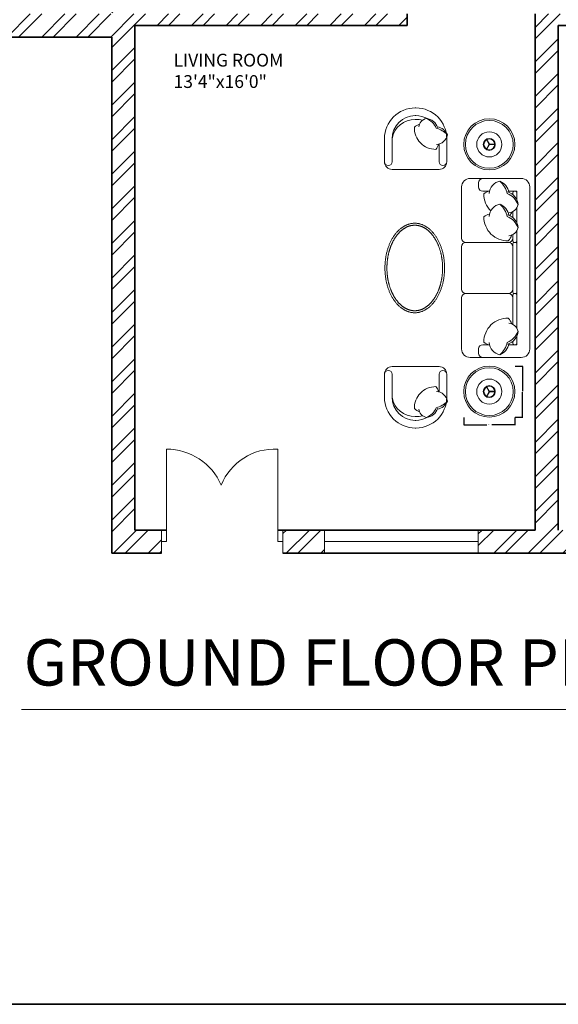
# Model space of a CAD drawing. Units: inches. Extents: x 1152 to 2588, y 1459 to 2618.
# Tile 2 of 17: x 1369 to 1579, y 1459 to 1843. Entities that reach past the tile are written whole.
import ezdxf

# ---------------------------------------------------------------- set-up
doc = ezdxf.new("R2010")
doc.units = ezdxf.units.IN
for name, color, linetype, lineweight in [('A-ANNO-DIMS', 2, 'Continuous', 18), ('A-ANNO-TEXT', 7, 'Continuous', 18), ('A-ANNO-TTLB', 7, 'Continuous', 35), ('A-AREA-IDEN', 7, 'Continuous', 18), ('A-DOOR', 4, 'Continuous', 18), ('A-FURN', 8, 'Continuous', 13), ('A-GLAZ', 4, 'Continuous', 18), ('A-WALL', 7, 'Continuous', 35), ('A-WALL-PATT', 8, 'Continuous', 13)]:
    doc.layers.add(name, color=color, linetype=linetype, lineweight=lineweight)
doc.styles.get("Standard").update_dxf_attribs({"font": 'arial.ttf'})
doc.dimstyles.get("Standard").update_dxf_attribs({"dimtxt": 0.18, "dimasz": 0.18, "dimexe": 0.18, "dimexo": 0.0625, "dimgap": 0.09, "dimtad": 0, "dimtih": 1, "dimtoh": 1, "dimdec": 4, "dimzin": 0, "dimdsep": 46, "dimtxsty": 'Standard', "dimcen": 0.09, "dimadec": 0, "dimazin": 0, "dimtfac": 1, "dimtdec": 4, "dimtofl": 0, "dimtmove": 0, "dimatfit": 3, "dimfxl": 1, "dimtolj": 1, "dimtzin": 0, "dimarcsym": 0})

# ---------------------------------------------------------------- blocks, each defined once
blk = doc.blocks.new('TABLE-ROUND-SIDE')
at = {"ltscale": 0.03}
for p, q in [((9.87, 9.91), (8.7, 11.94)), ((10.05, 10.01), (8.88, 12.04)), ((9.87, 10.01), (8.7, 7.99)), ((10.05, 9.91), (8.88, 7.88)), ((9.96, 10.07), (12.3, 10.07)), ((9.96, 9.86), (12.3, 9.86))]:
    blk.add_line(p, q, dxfattribs=at)
for radius in [9.96, 4.9, 2.34, 2.1]:
    blk.add_circle((9.96, 9.96), radius, dxfattribs=at)
blk.add_circle((9.96, 9.96), 9.3)
blk = doc.blocks.new('DOOR-DOUBLE-ENTRY')
for p, q in [((2, 4.5), (2, 40.5)), ((45.34, 4.5), (45.34, 40.5)), ((0, 9), (0, 0)), ((47.34, 9), (47.34, 0)), ((0, 0), (0, 4.5)), ((0, 4.5), (2, 4.5)), ((47.34, 4.5), (45.34, 4.5)), ((47.34, 0), (47.34, 4.5))]:
    blk.add_line(p, q)
for centre, radius, start, end in [((2, 17.3), 23.2, 23.3053, 90), ((44.08, 18.16), 22.37, 86.7789, 158.1829)]:
    blk.add_arc(centre, radius, start, end)
blk = doc.blocks.new('WIN-60-FRONT')
for p, q in [((0, 9), (0, 0)), ((60, 4.5), (60, 9)), ((60, 9), (60, 0)), ((0, 0), (0, 4.5)), ((0, 4.5), (48, 4.5)), ((48, 4.5), (60, 4.5))]:
    blk.add_line(p, q)
blk = doc.blocks.new('*D34')
at = {"layer": 'A-ANNO-DIMS', "color": 0, "lineweight": -2, "transparency": 16777216}
for p, q in [((1542.56, 1687.93), (1542.56, 1684.83)), ((1562.48, 1687.93), (1562.48, 1684.83)), ((1542.74, 1685.01), (1551.55, 1685.01)), ((1562.3, 1685.01), (1553.48, 1685.01))]:
    blk.add_line(p, q, dxfattribs=at)
at = {"layer": 'A-ANNO-DIMS', "color": 0, "transparency": 16777216}
for points in [[(1542.74, 1685.04), (1542.74, 1684.98), (1542.56, 1685.01)], [(1562.3, 1685.04), (1562.3, 1684.98), (1562.48, 1685.01)]]:
    blk.add_solid(points, dxfattribs=at)
at = {"layer": 'Defpoints', "color": 0, "transparency": 16777216}
for p in [(1542.56, 1688), (1562.48, 1688), (1562.48, 1685.01)]:
    blk.add_point(p, dxfattribs=at)
at = {"layer": 'A-ANNO-DIMS', "color": 0, "transparency": 16777216, "insert": (1552.52, 1685.01), "char_height": 0.18, "attachment_point": 5}
blk.add_mtext('\\A1;TABLE 20 TYP.', dxfattribs=at)
blk = doc.blocks.new('*D35')
at = {"layer": 'A-ANNO-DIMS', "color": 0, "lineweight": -2, "transparency": 16777216}
for p, q in [((1562.54, 1707.92), (1565.65, 1707.92)), ((1565.47, 1707.74), (1565.47, 1698.14)), ((1565.47, 1688.18), (1565.47, 1697.78)), ((1562.54, 1688), (1565.65, 1688))]:
    blk.add_line(p, q, dxfattribs=at)
at = {"layer": 'A-ANNO-DIMS', "color": 0, "transparency": 16777216}
for points in [[(1565.44, 1707.74), (1565.5, 1707.74), (1565.47, 1707.92)], [(1565.44, 1688.18), (1565.5, 1688.18), (1565.47, 1688)]]:
    blk.add_solid(points, dxfattribs=at)
at = {"layer": 'Defpoints', "color": 0, "transparency": 16777216}
for p in [(1562.48, 1707.92), (1565.47, 1707.92), (1562.48, 1688)]:
    blk.add_point(p, dxfattribs=at)
at = {"layer": 'A-ANNO-DIMS', "color": 0, "transparency": 16777216, "insert": (1565.47, 1697.96), "char_height": 0.18, "attachment_point": 5}
blk.add_mtext('\\A1;20 TYP.', dxfattribs=at)

msp = doc.modelspace()

# ---------------------------------------------------------------- hatches: boundary and pattern name
at = {"layer": 'A-WALL-PATT'}
h = msp.add_hatch(dxfattribs=at)
h.set_pattern_fill('ANSI32', color=256)
h.paths.add_polyline_path([(1408.9272, 2240.0458), (1276.4165, 2240.0458), (1276.4165, 2192.7491), (1285.4165, 2192.7491), (1285.4165, 2231.0458), (1369.4165, 2231.0458), (1369.4165, 2084.0458), (1526.9165, 2084.0458), (1526.9165, 2096.3728), (1524.6665, 2096.3728), (1522.4165, 2096.3728), (1522.4165, 2093.0458), (1378.4165, 2093.0458), (1378.4165, 2231.0458), (1408.9272, 2231.0458)])
h.paths.add_polyline_path([(1736.4165, 2240.0458), (1468.9272, 2240.0458), (1468.9272, 2231.0458), (1522.4165, 2231.0458), (1522.4165, 2127.3313), (1526.9165, 2127.3313), (1526.9165, 2231.0458), (1574.9165, 2231.0458), (1574.9165, 2188.0458), (1579.4165, 2188.0458), (1579.4165, 2231.0458), (1727.4165, 2231.0458), (1727.4165, 2183.9728), (1736.4165, 2183.9728)])
h.paths.add_polyline_path([(1285.4165, 2156.7491), (1276.4165, 2156.7491), (1276.4165, 2084.0458), (1285.4165, 2084.0458)], flags=17)
h.paths.add_polyline_path([(1285.4165, 2043.5458), (1445.4165, 2043.5458), (1445.4165, 1943.6503), (1454.4165, 1943.6503), (1454.4165, 2048.0458), (1276.4165, 2048.0458), (1276.4165, 2019.2077), (1280.9165, 2019.2077), (1285.4165, 2019.2077)])
h.paths.add_polyline_path([(1285.4165, 1959.2077), (1276.4165, 1959.2077), (1276.4165, 1891.1319), (1280.9165, 1891.1319), (1285.4165, 1891.1319), (1285.4165, 1901.0458), (1376.8505, 1901.0458), (1376.8505, 1903.2958), (1376.8505, 1905.5458), (1285.4165, 1905.5458)])
h.paths.add_polyline_path([(1518.4165, 1905.5458), (1399.2832, 1905.5458), (1399.2832, 1903.2958), (1399.2832, 1901.0458), (1405.4165, 1901.0458), (1405.4165, 1884.8579), (1409.9165, 1884.8579), (1409.9165, 1901.0458), (1513.9165, 1901.0458), (1513.9165, 1869.1706), (1518.4165, 1869.1706)])
h.paths.add_polyline_path([(1520.5229, 1845.0458), (1518.4165, 1845.0458), (1518.4165, 1849.2927), (1516.1665, 1849.2927), (1513.9165, 1849.2927), (1513.9165, 1845.0458), (1409.9165, 1845.0458), (1409.9165, 1860.8579), (1405.4165, 1860.8579), (1405.4165, 1845.0458), (1285.4165, 1845.0458), (1285.4165, 1867.1319), (1276.4165, 1867.1319), (1276.4165, 1635.0458), (1285.4165, 1635.0458), (1285.4165, 1836.0458), (1405.4165, 1836.0458), (1405.4165, 1635.0458), (1414.4165, 1635.0458), (1424.7277, 1635.0458), (1424.7277, 1639.5458), (1424.7277, 1644.0458), (1414.4165, 1644.0458), (1414.4165, 1836.0458), (1414.4165, 1840.5831), (1520.5229, 1840.5831)])
h.paths.add_polyline_path([(1579.4165, 1840.5458), (1583.4035, 1840.5458), (1583.4035, 1845.0458), (1579.4165, 1845.0458), (1570.4165, 1845.0458), (1570.4165, 1840.5831), (1570.4165, 1644.0458), (1548.2359, 1644.0458), (1548.2359, 1635.0458), (1611.2801, 1635.0458), (1611.2801, 1639.5458), (1611.2801, 1644.0458), (1579.4165, 1644.0458)])
h.paths.add_polyline_path([(1488.2359, 1644.0458), (1472.0663, 1644.0458), (1472.0663, 1635.0458), (1488.2359, 1635.0458), (1488.2359, 1639.5458)], flags=17)
h.paths.add_polyline_path([(1736.4165, 1701.1863), (1727.4165, 1701.1863), (1727.4165, 1644.0458), (1671.2801, 1644.0458), (1671.2801, 1635.0458), (1736.4165, 1635.0458)])
h.paths.add_polyline_path([(1736.4165, 2147.9728), (1727.4165, 2147.9728), (1727.4165, 2093.0458), (1579.4165, 2093.0458), (1574.9165, 2093.0458), (1574.9165, 1971.6501), (1579.4165, 1971.6501), (1579.4165, 2084.0458), (1727.4165, 2084.0458), (1727.4165, 2054.3847), (1736.4165, 2054.3847)])
h.paths.add_polyline_path([(1736.4165, 1994.3847), (1727.4165, 1994.3847), (1727.4165, 1911.3562), (1736.4165, 1911.3562)])
h.paths.add_polyline_path([(1736.4165, 1875.3562), (1727.4165, 1875.3562), (1727.4165, 1845.0458), (1617.1767, 1845.0458), (1617.1767, 1842.7958), (1617.1767, 1840.5458), (1618.9165, 1840.5458), (1618.9165, 1788.5458), (1618.9165, 1784.0458), (1627.8699, 1784.0458), (1627.8699, 1788.5458), (1623.4165, 1788.5458), (1623.4165, 1840.5458), (1727.4165, 1840.5458), (1727.4165, 1828.7619), (1736.4165, 1828.7619)])
h.paths.add_polyline_path([(1727.4165, 1938.0458), (1579.4165, 1938.0458), (1579.4165, 1942.7722), (1574.9165, 1942.7722), (1574.9165, 1929.0458), (1727.4165, 1929.0458)])

# ---------------------------------------------------------------- linework, layer by layer
at = {"layer": 'A-ANNO-TEXT'}
msp.add_line((1370.1295, 1574.1335), (1649.1589, 1574.1335), dxfattribs=at)
at = {"layer": 'A-ANNO-TTLB'}
msp.add_lwpolyline([(1152.3215, 2617.6685), (2587.6987, 2617.6685), (2587.6987, 1459.3148), (1152.3215, 1459.3148)], close=True, dxfattribs=at)
at = {"layer": 'A-FURN', "ltscale": 0.03}
for points in [[(1523.795, 1784.4921), (1514.6636, 1784.4921, -0.41421356), (1511.6697, 1787.486), (1511.6697, 1796.4677, -0.41421356), (1523.6453, 1808.4434), (1523.795, 1808.4434), (1523.9447, 1808.4434, -0.41421356), (1535.9204, 1796.4677), (1535.9204, 1787.486, -0.41421356), (1532.9265, 1784.4921), (1523.795, 1784.4921)], [(1523.795, 1707.7174), (1514.6636, 1707.7174, 0.41421356), (1511.6697, 1704.7235), (1511.6697, 1695.7417, 0.41421356), (1523.6453, 1683.7661), (1523.795, 1683.7661), (1523.9447, 1683.7661, 0.41421356), (1535.9204, 1695.7417), (1535.9204, 1704.7235, 0.41421356), (1532.9265, 1707.7174), (1523.795, 1707.7174)]]:
    msp.add_lwpolyline(points, format="xyb", dxfattribs=at)
at = {"layer": 'A-FURN'}
for points in [[(1514.6636, 1796.4677, -0.41421356), (1523.6453, 1805.4495), (1523.795, 1805.4495)], [(1514.6636, 1796.4677, -0.37271891), (1523.6453, 1803.9525), (1523.795, 1803.9525)], [(1528.4031, 1804.2648, 0.13059149), (1523.9447, 1805.4495), (1523.795, 1805.4495)], [(1526.4969, 1803.63, 0.07238424), (1523.9447, 1803.9525), (1523.795, 1803.9525)], [(1532.3945, 1800.7566, 0.30666349), (1527.9296, 1804.3248, 0.30632997), (1525.0128, 1801.0661, -0.87284716)], [(1536.1652, 1797.9789, 0.14772988), (1531.7901, 1800.5515, 0.21334276), (1527.9296, 1804.3248, 0.17866181)], [(1532.6303, 1794.2969, -0.16554063), (1531.7043, 1792.319, -0.42598917), (1523.2971, 1800.8945, -0.12152332), (1525.2928, 1802.0765, 7.11546429)], [(1531.8758, 1794.2056, 0.35677236), (1536.1652, 1797.9789, 0.24954205), (1532.2786, 1801.0883, -9.61688035)], [(1514.6636, 1796.4679), (1514.6636, 1787.486, -0.41421356), (1513.1666, 1785.989), (1513.1666, 1785.989, -0.41421356), (1511.6697, 1787.486)], [(1532.9265, 1794.3689), (1532.9265, 1787.486, 0.41421356), (1534.4234, 1785.989), (1534.4234, 1785.989, 0.41421356), (1535.9204, 1787.486)], [(1552.5995, 1775.9894), (1550.0272, 1775.9894, -0.41421356), (1548.3669, 1777.6497), (1548.3669, 1779.31, -0.41421356), (1550.0272, 1780.9702)], [(1552.499, 1775.1563, -0.35677236), (1556.6839, 1779.9136, -0.24954205), (1560.1326, 1775.603, 9.61688035)], [(1556.6839, 1779.9136, -0.14772988), (1559.5372, 1775.0611, -0.21334276), (1563.7221, 1770.7795, -0.17866181)], [(1552.6003, 1775.9931, 0.16554063), (1550.4066, 1774.966, 0.20023115), (1553.0783, 1768.3753, 0.12152332)], [(1559.7646, 1775.7315, -0.30666349), (1563.7221, 1770.7795, -0.30632997), (1560.1079, 1767.5445, 0.87284716)], [(1563.3092, 1772.4967), (1563.3092, 1775.9894), (1560.0464, 1775.9894, -0.41421356)], [(1561.649, 1774.7225), (1561.649, 1775.3253, -0.41421356), (1562.3131, 1775.9894), (1562.6451, 1775.9894, -0.41421356), (1563.3092, 1775.3253)], [(1563.3092, 1775.3253), (1563.3092, 1772.4967, -0.41421356)], [(1552.499, 1766.2125, -0.35677236), (1556.6839, 1770.9698, -0.24954205), (1560.1326, 1766.6592, 9.61688035)], [(1556.6839, 1770.9698, -0.14772988), (1559.5372, 1766.1173, -0.21334276), (1563.7221, 1761.8358, -0.17866181)], [(1561.649, 1765.7787), (1561.649, 1768.0629, -0.41421356)], [(1563.3092, 1769.7346), (1563.3092, 1763.5529, -0.41421356)], [(1552.6003, 1767.0493, 0.16554063), (1550.4066, 1766.0222, 0.42598917), (1559.9177, 1756.6978, 0.12152332), (1561.2286, 1758.9113, -7.11546429)], [(1559.7646, 1766.7877, -0.30666349), (1563.7221, 1761.8358, -0.30632997), (1560.1079, 1758.6008, 0.87284716)], [(1560.5795, 1766.4631, 0.07186538), (1561.2286, 1767.855, -7.11546429)], [(1563.3092, 1760.7909), (1563.3092, 1756.7304, -0.41421356), (1562.6451, 1756.0663), (1562.3131, 1756.0663, -0.41421356), (1561.649, 1756.7304), (1561.649, 1759.1191, -0.41421356)], [(1561.649, 1757.7266, -0.41421356), (1559.9887, 1756.0663), (1543.3861, 1756.0663, -0.41421356)], [(1561.649, 1754.406, 0.41421356), (1559.9887, 1756.0663)], [(1561.649, 1737.8034, -0.41421356), (1559.9887, 1736.1432)], [(1561.649, 1734.4829, 0.41421356), (1559.9887, 1736.1432), (1543.3861, 1736.1432, 0.41421356)], [(1563.3092, 1722.4748), (1563.3092, 1735.4791, 0.41421356), (1562.6451, 1736.1432), (1562.3131, 1736.1432, 0.41421356), (1561.649, 1735.4791), (1561.649, 1724.1466, 0.41421356)], [(1552.6003, 1716.2164, -0.16554063), (1550.4066, 1717.2435, -0.42598917), (1559.9177, 1726.5679, -0.12152332), (1561.2286, 1724.3544, 7.11546429)], [(1559.7646, 1716.478, 0.30666349), (1563.7221, 1721.43, 0.30632997), (1560.1079, 1724.6649, -0.87284716)], [(1556.6839, 1712.2959, 0.14772988), (1559.5372, 1717.1484, 0.21334276), (1563.7221, 1721.43, 0.17866181)], [(1563.3092, 1716.8841), (1563.3092, 1719.7128, 0.41421356)], [(1550.0272, 1711.2392, -0.41421356), (1548.3669, 1712.8995), (1548.3669, 1714.5598, -0.41421356), (1550.0272, 1716.22), (1552.5995, 1716.22)], [(1552.499, 1717.0532, 0.35677236), (1556.6839, 1712.2959, 0.24954205), (1560.1326, 1716.6065, -9.61688035)], [(1561.649, 1717.487), (1561.649, 1716.8841, 0.41421356), (1562.3131, 1716.22), (1562.6451, 1716.22, 0.41421356), (1563.3092, 1716.8841)], [(1514.6636, 1695.7416), (1514.6636, 1704.7235, 0.41421356), (1513.1666, 1706.2204), (1513.1666, 1706.2204, 0.41421356), (1511.6697, 1704.7235)], [(1532.9265, 1697.8406), (1532.9265, 1704.7235, -0.41421356), (1534.4234, 1706.2204), (1534.4234, 1706.2204, -0.41421356), (1535.9204, 1704.7235)], [(1532.6303, 1697.9126, 0.16554063), (1531.7043, 1699.8905, 0.42598917), (1523.2971, 1691.3149, 0.12152332), (1525.2928, 1690.1329, -7.11546429)], [(1514.6636, 1695.7417, 0.37271891), (1523.6453, 1688.257), (1523.795, 1688.257)], [(1514.6636, 1695.7417, 0.41421356), (1523.6453, 1686.76), (1523.795, 1686.76)], [(1531.8758, 1698.0039, -0.35677236), (1536.1652, 1694.2306, -0.24954205), (1532.2786, 1691.1211, 9.61688035)], [(1532.3945, 1691.4529, -0.30666349), (1527.9296, 1687.8847, -0.30632997), (1525.0128, 1691.1434, 0.87284716)], [(1536.1652, 1694.2306, -0.14772988), (1531.7901, 1691.6579, -0.21334276), (1527.9296, 1687.8847, -0.17866181)], [(1526.4969, 1688.5795, -0.07238424), (1523.9447, 1688.257), (1523.795, 1688.257)], [(1528.4031, 1687.9446, -0.13059149), (1523.9447, 1686.76), (1523.795, 1686.76)]]:
    msp.add_lwpolyline(points, format="xyb", dxfattribs=at)
at = {"layer": 'A-FURN', "ltscale": 0.03}
msp.add_lwpolyline([(1545.0464, 1711.2392, -0.41421356), (1541.7258, 1714.5598), (1541.7258, 1734.4829, -0.41421356), (1543.3861, 1736.1432, -0.41421356), (1541.7258, 1737.8034), (1541.7258, 1754.406, -0.41421356), (1543.3861, 1756.0663, -0.41421356), (1541.7258, 1757.7266), (1541.7258, 1777.6497, -0.41421356), (1545.0464, 1780.9702), (1564.9695, 1780.9702, -0.41421356), (1568.29, 1777.6497), (1568.29, 1714.5598, -0.41421356), (1564.9695, 1711.2392)], format="xyb", close=True, dxfattribs=at)
at = {"layer": 'A-FURN'}
for points in [[(1563.3092, 1763.5529), (1563.3092, 1769.7346)], [(1563.3092, 1722.4748), (1563.3092, 1760.7909)], [(1560.0464, 1716.22), (1563.3092, 1716.22), (1563.3092, 1719.7128)]]:
    msp.add_lwpolyline(points, dxfattribs=at)
msp.add_lwpolyline([(1563.3092, 1755.4022), (1563.3092, 1736.8073, -0.41421356), (1562.6451, 1736.1432), (1562.3131, 1736.1432, -0.41421356), (1561.649, 1736.8073), (1561.649, 1755.4022, -0.41421356), (1562.3131, 1756.0663), (1562.6451, 1756.0663, -0.41421356)], format="xyb", close=True, dxfattribs=at)
at = {"layer": 'A-FURN', "ltscale": 0.03}
msp.add_polyline3d([(1523.463, 1728.672, 0), (1523.6829, 1728.6751, 0), (1523.9028, 1728.6845, 0), (1524.1225, 1728.7001, 0), (1524.3419, 1728.7219, 0), (1524.5611, 1728.75, 0), (1524.7798, 1728.7843, 0), (1524.9981, 1728.8247, 0), (1525.2158, 1728.8714, 0), (1525.4329, 1728.9243, 0), (1525.6493, 1728.9833, 0), (1525.8649, 1729.0484, 0), (1526.0797, 1729.1196, 0), (1526.2935, 1729.1969, 0), (1526.5063, 1729.2803, 0), (1526.718, 1729.3697, 0), (1526.9286, 1729.4651, 0), (1527.1379, 1729.5665, 0), (1527.3459, 1729.6737, 0), (1527.5525, 1729.7869, 0), (1527.7576, 1729.9059, 0), (1527.9612, 1730.0307, 0), (1528.1632, 1730.1613, 0), (1528.3635, 1730.2976, 0), (1528.562, 1730.4395, 0), (1528.7588, 1730.5871, 0), (1528.9536, 1730.7402, 0), (1529.1464, 1730.8988, 0), (1529.3373, 1731.0628, 0), (1529.526, 1731.2323, 0), (1529.7125, 1731.407, 0), (1529.8968, 1731.5871, 0), (1530.0788, 1731.7723, 0), (1530.2585, 1731.9627, 0), (1530.4357, 1732.1581, 0), (1530.6104, 1732.3585, 0), (1530.7825, 1732.5639, 0), (1530.952, 1732.7741, 0), (1531.1189, 1732.989, 0), (1531.283, 1733.2087, 0), (1531.4443, 1733.433, 0), (1531.6027, 1733.6618, 0), (1531.7582, 1733.8951, 0), (1531.9108, 1734.1328, 0), (1532.0603, 1734.3747, 0), (1532.2068, 1734.6209, 0), (1532.3501, 1734.8711, 0), (1532.4902, 1735.1254, 0), (1532.6271, 1735.3836, 0), (1532.7607, 1735.6457, 0), (1532.891, 1735.9115, 0), (1533.0179, 1736.1809, 0), (1533.1414, 1736.4539, 0), (1533.2614, 1736.7304, 0), (1533.378, 1737.0102, 0), (1533.4909, 1737.2933, 0), (1533.6003, 1737.5795, 0), (1533.706, 1737.8688, 0), (1533.8081, 1738.1611, 0), (1533.9065, 1738.4561, 0), (1534.0011, 1738.754, 0), (1534.0919, 1739.0544, 0), (1534.179, 1739.3574, 0), (1534.2622, 1739.6628, 0), (1534.3415, 1739.9705, 0), (1534.417, 1740.2804, 0), (1534.4885, 1740.5924, 0), (1534.5561, 1740.9063, 0), (1534.6197, 1741.2222, 0), (1534.6793, 1741.5397, 0), (1534.7348, 1741.8589, 0), (1534.7864, 1742.1797, 0), (1534.8339, 1742.5018, 0), (1534.8773, 1742.8252, 0), (1534.9166, 1743.1498, 0), (1534.9519, 1743.4755, 0), (1534.983, 1743.8021, 0), (1535.01, 1744.1295, 0), (1535.0328, 1744.4576, 0), (1535.0515, 1744.7863, 0), (1535.0661, 1745.1155, 0), (1535.0765, 1745.4451, 0), (1535.0827, 1745.7748, 0), (1535.0848, 1746.1047, 0), (1535.0827, 1746.4346, 0), (1535.0765, 1746.7644, 0), (1535.0661, 1747.094, 0), (1535.0515, 1747.4232, 0), (1535.0328, 1747.7519, 0), (1535.01, 1748.08, 0), (1534.983, 1748.4074, 0), (1534.9519, 1748.734, 0), (1534.9166, 1749.0597, 0), (1534.8773, 1749.3843, 0), (1534.8339, 1749.7077, 0), (1534.7864, 1750.0298, 0), (1534.7348, 1750.3505, 0), (1534.6793, 1750.6698, 0), (1534.6197, 1750.9873, 0), (1534.5561, 1751.3031, 0), (1534.4885, 1751.6171, 0), (1534.417, 1751.9291, 0), (1534.3415, 1752.239, 0), (1534.2622, 1752.5467, 0), (1534.179, 1752.8521, 0), (1534.0919, 1753.1551, 0), (1534.0011, 1753.4555, 0), (1533.9065, 1753.7533, 0), (1533.8081, 1754.0484, 0), (1533.706, 1754.3407, 0), (1533.6003, 1754.6299, 0), (1533.4909, 1754.9162, 0), (1533.378, 1755.1993, 0), (1533.2614, 1755.4791, 0), (1533.1414, 1755.7555, 0), (1533.0179, 1756.0285, 0), (1532.891, 1756.298, 0), (1532.7607, 1756.5638, 0), (1532.6271, 1756.8258, 0), (1532.4902, 1757.0841, 0), (1532.3501, 1757.3383, 0), (1532.2068, 1757.5886, 0), (1532.0603, 1757.8348, 0), (1531.9108, 1758.0767, 0), (1531.7582, 1758.3144, 0), (1531.6027, 1758.5476, 0), (1531.4443, 1758.7765, 0), (1531.283, 1759.0008, 0), (1531.1189, 1759.2204, 0), (1530.952, 1759.4354, 0), (1530.7825, 1759.6456, 0), (1530.6104, 1759.8509, 0), (1530.4357, 1760.0514, 0), (1530.2585, 1760.2468, 0), (1530.0788, 1760.4372, 0), (1529.8968, 1760.6224, 0), (1529.7125, 1760.8024, 0), (1529.526, 1760.9772, 0), (1529.3373, 1761.1466, 0), (1529.1464, 1761.3107, 0), (1528.9536, 1761.4693, 0), (1528.7588, 1761.6224, 0), (1528.562, 1761.77, 0), (1528.3635, 1761.9119, 0), (1528.1632, 1762.0482, 0), (1527.9612, 1762.1787, 0), (1527.7576, 1762.3036, 0), (1527.5525, 1762.4226, 0), (1527.3459, 1762.5357, 0), (1527.1379, 1762.643, 0), (1526.9286, 1762.7444, 0), (1526.718, 1762.8398, 0), (1526.5063, 1762.9292, 0), (1526.2935, 1763.0125, 0), (1526.0797, 1763.0899, 0), (1525.8649, 1763.1611, 0), (1525.6493, 1763.2262, 0), (1525.4329, 1763.2852, 0), (1525.2158, 1763.3381, 0), (1524.9981, 1763.3847, 0), (1524.7798, 1763.4252, 0), (1524.5611, 1763.4595, 0), (1524.3419, 1763.4876, 0), (1524.1225, 1763.5094, 0), (1523.9028, 1763.525, 0), (1523.6829, 1763.5344, 0), (1523.463, 1763.5375, 0), (1523.243, 1763.5344, 0), (1523.0232, 1763.525, 0), (1522.8035, 1763.5094, 0), (1522.584, 1763.4876, 0), (1522.3649, 1763.4595, 0), (1522.1461, 1763.4252, 0), (1521.9279, 1763.3847, 0), (1521.7101, 1763.3381, 0), (1521.493, 1763.2852, 0), (1521.2766, 1763.2262, 0), (1521.061, 1763.1611, 0), (1520.8463, 1763.0899, 0), (1520.6324, 1763.0125, 0), (1520.4196, 1762.9292, 0), (1520.2079, 1762.8398, 0), (1519.9974, 1762.7444, 0), (1519.7881, 1762.643, 0), (1519.5801, 1762.5357, 0), (1519.3735, 1762.4226, 0), (1519.1683, 1762.3036, 0), (1518.9647, 1762.1787, 0), (1518.7628, 1762.0482, 0), (1518.5625, 1761.9119, 0), (1518.3639, 1761.77, 0), (1518.1672, 1761.6224, 0), (1517.9724, 1761.4693, 0), (1517.7795, 1761.3107, 0), (1517.5887, 1761.1466, 0), (1517.4, 1760.9772, 0), (1517.2134, 1760.8024, 0), (1517.0291, 1760.6224, 0), (1516.8471, 1760.4372, 0), (1516.6675, 1760.2468, 0), (1516.4903, 1760.0514, 0), (1516.3156, 1759.8509, 0), (1516.1434, 1759.6456, 0), (1515.9739, 1759.4354, 0), (1515.8071, 1759.2204, 0), (1515.643, 1759.0008, 0), (1515.4817, 1758.7765, 0), (1515.3232, 1758.5476, 0), (1515.1677, 1758.3144, 0), (1515.0152, 1758.0767, 0), (1514.8656, 1757.8348, 0), (1514.7192, 1757.5886, 0), (1514.5759, 1757.3383, 0), (1514.4357, 1757.0841, 0), (1514.2988, 1756.8258, 0), (1514.1652, 1756.5638, 0), (1514.0349, 1756.298, 0), (1513.908, 1756.0285, 0), (1513.7845, 1755.7555, 0), (1513.6645, 1755.4791, 0), (1513.548, 1755.1993, 0), (1513.435, 1754.9162, 0), (1513.3257, 1754.6299, 0), (1513.2199, 1754.3407, 0), (1513.1179, 1754.0484, 0), (1513.0195, 1753.7533, 0), (1512.9249, 1753.4555, 0), (1512.834, 1753.1551, 0), (1512.747, 1752.8521, 0), (1512.6638, 1752.5467, 0), (1512.5844, 1752.239, 0), (1512.509, 1751.9291, 0), (1512.4375, 1751.6171, 0), (1512.3699, 1751.3031, 0), (1512.3063, 1750.9873, 0), (1512.2467, 1750.6698, 0), (1512.1911, 1750.3505, 0), (1512.1396, 1750.0298, 0), (1512.0921, 1749.7077, 0), (1512.0487, 1749.3843, 0), (1512.0093, 1749.0597, 0), (1511.9741, 1748.734, 0), (1511.943, 1748.4074, 0), (1511.916, 1748.08, 0), (1511.8931, 1747.7519, 0), (1511.8744, 1747.4232, 0), (1511.8599, 1747.094, 0), (1511.8495, 1746.7644, 0), (1511.8432, 1746.4346, 0), (1511.8411, 1746.1047, 0), (1511.8432, 1745.7748, 0), (1511.8495, 1745.4451, 0), (1511.8599, 1745.1155, 0), (1511.8744, 1744.7863, 0), (1511.8931, 1744.4576, 0), (1511.916, 1744.1295, 0), (1511.943, 1743.8021, 0), (1511.9741, 1743.4755, 0), (1512.0093, 1743.1498, 0), (1512.0487, 1742.8252, 0), (1512.0921, 1742.5018, 0), (1512.1396, 1742.1797, 0), (1512.1911, 1741.8589, 0), (1512.2467, 1741.5397, 0), (1512.3063, 1741.2222, 0), (1512.3699, 1740.9063, 0), (1512.4375, 1740.5924, 0), (1512.509, 1740.2804, 0), (1512.5844, 1739.9705, 0), (1512.6638, 1739.6628, 0), (1512.747, 1739.3574, 0), (1512.834, 1739.0544, 0), (1512.9249, 1738.754, 0), (1513.0195, 1738.4561, 0), (1513.1179, 1738.1611, 0), (1513.2199, 1737.8688, 0), (1513.3257, 1737.5795, 0), (1513.435, 1737.2933, 0), (1513.548, 1737.0102, 0), (1513.6645, 1736.7304, 0), (1513.7845, 1736.4539, 0), (1513.908, 1736.1809, 0), (1514.0349, 1735.9115, 0), (1514.1652, 1735.6457, 0), (1514.2988, 1735.3836, 0), (1514.4357, 1735.1254, 0), (1514.5759, 1734.8711, 0), (1514.7192, 1734.6209, 0), (1514.8656, 1734.3747, 0), (1515.0152, 1734.1328, 0), (1515.1677, 1733.8951, 0), (1515.3232, 1733.6618, 0), (1515.4817, 1733.433, 0), (1515.643, 1733.2087, 0), (1515.8071, 1732.989, 0), (1515.9739, 1732.7741, 0), (1516.1434, 1732.5639, 0), (1516.3156, 1732.3585, 0), (1516.4903, 1732.1581, 0), (1516.6675, 1731.9627, 0), (1516.8471, 1731.7723, 0), (1517.0291, 1731.5871, 0), (1517.2134, 1731.407, 0), (1517.4, 1731.2323, 0), (1517.5887, 1731.0628, 0), (1517.7795, 1730.8988, 0), (1517.9724, 1730.7402, 0), (1518.1672, 1730.5871, 0), (1518.3639, 1730.4395, 0), (1518.5625, 1730.2976, 0), (1518.7628, 1730.1613, 0), (1518.9647, 1730.0307, 0), (1519.1683, 1729.9059, 0), (1519.3735, 1729.7869, 0), (1519.5801, 1729.6737, 0), (1519.7881, 1729.5665, 0), (1519.9974, 1729.4651, 0), (1520.2079, 1729.3697, 0), (1520.4196, 1729.2803, 0), (1520.6324, 1729.1969, 0), (1520.8463, 1729.1196, 0), (1521.061, 1729.0484, 0), (1521.2766, 1728.9833, 0), (1521.493, 1728.9243, 0), (1521.7101, 1728.8714, 0), (1521.9279, 1728.8247, 0), (1522.1461, 1728.7843, 0), (1522.3649, 1728.75, 0), (1522.584, 1728.7219, 0), (1522.8035, 1728.7001, 0), (1523.0232, 1728.6845, 0), (1523.243, 1728.6751, 0), (1523.463, 1728.672, 0)], dxfattribs=at)
at = {"layer": 'A-FURN'}
msp.add_polyline3d([(1523.463, 1729.4468, 0), (1523.5818, 1729.4478, 0), (1523.7012, 1729.4509, 0), (1523.8212, 1729.456, 0), (1523.9416, 1729.4632, 0), (1524.0626, 1729.4726, 0), (1524.184, 1729.4841, 0), (1524.3059, 1729.4978, 0), (1524.4283, 1729.5138, 0), (1524.551, 1729.5319, 0), (1524.6742, 1729.5523, 0), (1524.7978, 1729.575, 0), (1524.9218, 1729.6001, 0), (1525.0462, 1729.6274, 0), (1525.1709, 1729.6572, 0), (1525.2959, 1729.6893, 0), (1525.4212, 1729.7239, 0), (1525.5469, 1729.7609, 0), (1525.6728, 1729.8004, 0), (1525.799, 1729.8424, 0), (1525.9254, 1729.8869, 0), (1526.0521, 1729.934, 0), (1526.179, 1729.9837, 0), (1526.306, 1730.036, 0), (1526.4331, 1730.091, 0), (1526.5604, 1730.1486, 0), (1526.6876, 1730.2089, 0), (1526.8149, 1730.2717, 0), (1526.9421, 1730.3373, 0), (1527.0693, 1730.4055, 0), (1527.1964, 1730.4763, 0), (1527.3233, 1730.5498, 0), (1527.45, 1730.626, 0), (1527.5765, 1730.7048, 0), (1527.7028, 1730.7863, 0), (1527.8288, 1730.8705, 0), (1527.9544, 1730.9574, 0), (1528.0796, 1731.0469, 0), (1528.2045, 1731.1392, 0), (1528.3289, 1731.2341, 0), (1528.4528, 1731.3317, 0), (1528.5761, 1731.432, 0), (1528.699, 1731.5351, 0), (1528.8212, 1731.641, 0), (1528.9428, 1731.7499, 0), (1529.0637, 1731.8615, 0), (1529.184, 1731.976, 0), (1529.3036, 1732.0933, 0), (1529.4224, 1732.2133, 0), (1529.5404, 1732.336, 0), (1529.6576, 1732.4613, 0), (1529.774, 1732.5893, 0), (1529.8895, 1732.7198, 0), (1530.0041, 1732.8528, 0), (1530.1177, 1732.9884, 0), (1530.2304, 1733.1263, 0), (1530.3421, 1733.2667, 0), (1530.4527, 1733.4095, 0), (1530.5623, 1733.5545, 0), (1530.6708, 1733.7019, 0), (1530.7782, 1733.8515, 0), (1530.8844, 1734.0033, 0), (1530.9894, 1734.1573, 0), (1531.0931, 1734.3134, 0), (1531.1957, 1734.4716, 0), (1531.2969, 1734.6318, 0), (1531.3968, 1734.794, 0), (1531.4954, 1734.9582, 0), (1531.5925, 1735.1243, 0), (1531.6883, 1735.2923, 0), (1531.7826, 1735.4622, 0), (1531.8754, 1735.6338, 0), (1531.9668, 1735.8072, 0), (1532.0566, 1735.9823, 0), (1532.1448, 1736.1591, 0), (1532.2314, 1736.3375, 0), (1532.3163, 1736.5175, 0), (1532.3996, 1736.6991, 0), (1532.4812, 1736.8821, 0), (1532.5611, 1737.0667, 0), (1532.6392, 1737.2527, 0), (1532.7155, 1737.4401, 0), (1532.79, 1737.6288, 0), (1532.8626, 1737.8189, 0), (1532.9333, 1738.0099, 0), (1533.0021, 1738.2016, 0), (1533.0691, 1738.3937, 0), (1533.1343, 1738.5864, 0), (1533.1975, 1738.7795, 0), (1533.259, 1738.9732, 0), (1533.3186, 1739.1673, 0), (1533.3763, 1739.3618, 0), (1533.4323, 1739.5568, 0), (1533.4864, 1739.7523, 0), (1533.5387, 1739.9481, 0), (1533.5893, 1740.1444, 0), (1533.638, 1740.3411, 0), (1533.685, 1740.5381, 0), (1533.7302, 1740.7355, 0), (1533.7736, 1740.9333, 0), (1533.8153, 1741.1313, 0), (1533.8552, 1741.3298, 0), (1533.8934, 1741.5285, 0), (1533.9298, 1741.7275, 0), (1533.9646, 1741.9268, 0), (1533.9976, 1742.1264, 0), (1534.0289, 1742.3263, 0), (1534.0585, 1742.5264, 0), (1534.0864, 1742.7267, 0), (1534.1126, 1742.9273, 0), (1534.1372, 1743.128, 0), (1534.1601, 1743.329, 0), (1534.1813, 1743.5301, 0), (1534.2009, 1743.7314, 0), (1534.2188, 1743.9329, 0), (1534.2351, 1744.1345, 0), (1534.2498, 1744.3362, 0), (1534.2629, 1744.538, 0), (1534.2743, 1744.74, 0), (1534.2842, 1744.942, 0), (1534.2924, 1745.1441, 0), (1534.2991, 1745.3463, 0), (1534.3041, 1745.5485, 0), (1534.3076, 1745.7507, 0), (1534.3096, 1745.953, 0), (1534.31, 1746.1553, 0), (1534.3088, 1746.3576, 0), (1534.3061, 1746.5599, 0), (1534.3018, 1746.7621, 0), (1534.2959, 1746.9643, 0), (1534.2885, 1747.1664, 0), (1534.2794, 1747.3685, 0), (1534.2688, 1747.5705, 0), (1534.2565, 1747.7724, 0), (1534.2427, 1747.9742, 0), (1534.2272, 1748.1758, 0), (1534.2101, 1748.3774, 0), (1534.1913, 1748.5787, 0), (1534.1709, 1748.78, 0), (1534.1489, 1748.981, 0), (1534.1251, 1749.1819, 0), (1534.0997, 1749.3825, 0), (1534.0727, 1749.583, 0), (1534.0439, 1749.7832, 0), (1534.0134, 1749.9832, 0), (1533.9813, 1750.1829, 0), (1533.9474, 1750.3823, 0), (1533.9118, 1750.5815, 0), (1533.8745, 1750.7804, 0), (1533.8354, 1750.979, 0), (1533.7946, 1751.1772, 0), (1533.7521, 1751.3751, 0), (1533.7078, 1751.5727, 0), (1533.6617, 1751.7699, 0), (1533.6139, 1751.9668, 0), (1533.5642, 1752.1632, 0), (1533.5128, 1752.3593, 0), (1533.4596, 1752.555, 0), (1533.4045, 1752.7502, 0), (1533.3477, 1752.945, 0), (1533.289, 1753.1393, 0), (1533.2285, 1753.3332, 0), (1533.1661, 1753.5266, 0), (1533.1019, 1753.7195, 0), (1533.0359, 1753.9119, 0), (1532.968, 1754.1038, 0), (1532.8982, 1754.2951, 0), (1532.8265, 1754.4858, 0), (1532.753, 1754.6752, 0), (1532.6776, 1754.8633, 0), (1532.6004, 1755.05, 0), (1532.5214, 1755.2352, 0), (1532.4406, 1755.4191, 0), (1532.3582, 1755.6014, 0), (1532.2741, 1755.7822, 0), (1532.1883, 1755.9614, 0), (1532.1009, 1756.139, 0), (1532.0119, 1756.315, 0), (1531.9213, 1756.4892, 0), (1531.8292, 1756.6617, 0), (1531.7356, 1756.8325, 0), (1531.6406, 1757.0014, 0), (1531.5441, 1757.1684, 0), (1531.4462, 1757.3336, 0), (1531.347, 1757.4968, 0), (1531.2464, 1757.658, 0), (1531.1446, 1757.8172, 0), (1531.0414, 1757.9744, 0), (1530.937, 1758.1294, 0), (1530.8314, 1758.2823, 0), (1530.7246, 1758.433, 0), (1530.6167, 1758.5815, 0), (1530.5077, 1758.7278, 0), (1530.3976, 1758.8717, 0), (1530.2864, 1759.0132, 0), (1530.1742, 1759.1524, 0), (1530.061, 1759.2892, 0), (1529.9469, 1759.4235, 0), (1529.8319, 1759.5553, 0), (1529.7159, 1759.6845, 0), (1529.5991, 1759.8112, 0), (1529.4815, 1759.9352, 0), (1529.3631, 1760.0565, 0), (1529.2439, 1760.1752, 0), (1529.124, 1760.291, 0), (1529.0034, 1760.4041, 0), (1528.8821, 1760.5144, 0), (1528.7601, 1760.6218, 0), (1528.6376, 1760.7263, 0), (1528.5145, 1760.8279, 0), (1528.3909, 1760.9269, 0), (1528.2667, 1761.0232, 0), (1528.1421, 1761.1168, 0), (1528.0171, 1761.2076, 0), (1527.8916, 1761.2958, 0), (1527.7658, 1761.3814, 0), (1527.6397, 1761.4642, 0), (1527.5133, 1761.5444, 0), (1527.3867, 1761.6219, 0), (1527.2599, 1761.6967, 0), (1527.1329, 1761.7689, 0), (1527.0057, 1761.8384, 0), (1526.8785, 1761.9053, 0), (1526.7513, 1761.9695, 0), (1526.624, 1762.0311, 0), (1526.4967, 1762.09, 0), (1526.3695, 1762.1463, 0), (1526.2425, 1762.1999, 0), (1526.1155, 1762.2509, 0), (1525.9887, 1762.2993, 0), (1525.8622, 1762.3451, 0), (1525.7358, 1762.3884, 0), (1525.6098, 1762.4291, 0), (1525.484, 1762.4674, 0), (1525.3585, 1762.5032, 0), (1525.2333, 1762.5365, 0), (1525.1085, 1762.5675, 0), (1524.9839, 1762.596, 0), (1524.8598, 1762.6222, 0), (1524.736, 1762.6461, 0), (1524.6126, 1762.6676, 0), (1524.4896, 1762.6869, 0), (1524.367, 1762.704, 0), (1524.2449, 1762.7188, 0), (1524.1232, 1762.7314, 0), (1524.002, 1762.7418, 0), (1523.8813, 1762.7501, 0), (1523.7611, 1762.7563, 0), (1523.6415, 1762.7604, 0), (1523.5223, 1762.7624, 0), (1523.4036, 1762.7624, 0), (1523.2845, 1762.7604, 0), (1523.1648, 1762.7563, 0), (1523.0446, 1762.7501, 0), (1522.9239, 1762.7418, 0), (1522.8027, 1762.7314, 0), (1522.681, 1762.7188, 0), (1522.5589, 1762.704, 0), (1522.4364, 1762.6869, 0), (1522.3134, 1762.6676, 0), (1522.19, 1762.6461, 0), (1522.0662, 1762.6222, 0), (1521.942, 1762.596, 0), (1521.8175, 1762.5675, 0), (1521.6926, 1762.5365, 0), (1521.5674, 1762.5032, 0), (1521.4419, 1762.4674, 0), (1521.3162, 1762.4291, 0), (1521.1901, 1762.3884, 0), (1521.0638, 1762.3451, 0), (1520.9372, 1762.2993, 0), (1520.8105, 1762.2509, 0), (1520.6835, 1762.1999, 0), (1520.5564, 1762.1463, 0), (1520.4292, 1762.09, 0), (1520.302, 1762.0311, 0), (1520.1747, 1761.9695, 0), (1520.0474, 1761.9053, 0), (1519.9202, 1761.8384, 0), (1519.7931, 1761.7689, 0), (1519.6661, 1761.6967, 0), (1519.5393, 1761.6219, 0), (1519.4126, 1761.5444, 0), (1519.2862, 1761.4642, 0), (1519.1601, 1761.3814, 0), (1519.0343, 1761.2958, 0), (1518.9089, 1761.2076, 0), (1518.7838, 1761.1168, 0), (1518.6592, 1761.0232, 0), (1518.5351, 1760.9269, 0), (1518.4114, 1760.8279, 0), (1518.2883, 1760.7263, 0), (1518.1658, 1760.6218, 0), (1518.0439, 1760.5144, 0), (1517.9226, 1760.4041, 0), (1517.802, 1760.291, 0), (1517.6821, 1760.1752, 0), (1517.5629, 1760.0565, 0), (1517.4445, 1759.9352, 0), (1517.3268, 1759.8112, 0), (1517.21, 1759.6845, 0), (1517.0941, 1759.5553, 0), (1516.979, 1759.4235, 0), (1516.8649, 1759.2892, 0), (1516.7518, 1759.1524, 0), (1516.6396, 1759.0132, 0), (1516.5284, 1758.8717, 0), (1516.4183, 1758.7278, 0), (1516.3092, 1758.5815, 0), (1516.2013, 1758.433, 0), (1516.0945, 1758.2823, 0), (1515.9889, 1758.1294, 0), (1515.8846, 1757.9744, 0), (1515.7814, 1757.8172, 0), (1515.6795, 1757.658, 0), (1515.5789, 1757.4968, 0), (1515.4797, 1757.3336, 0), (1515.3818, 1757.1684, 0), (1515.2854, 1757.0014, 0), (1515.1903, 1756.8325, 0), (1515.0967, 1756.6617, 0), (1515.0046, 1756.4892, 0), (1514.9141, 1756.315, 0), (1514.8251, 1756.139, 0), (1514.7377, 1755.9614, 0), (1514.6519, 1755.7822, 0), (1514.5678, 1755.6014, 0), (1514.4853, 1755.4191, 0), (1514.4046, 1755.2352, 0), (1514.3256, 1755.05, 0), (1514.2484, 1754.8633, 0), (1514.173, 1754.6752, 0), (1514.0995, 1754.4858, 0), (1514.0278, 1754.2951, 0), (1513.958, 1754.1038, 0), (1513.8901, 1753.9119, 0), (1513.824, 1753.7195, 0), (1513.7598, 1753.5266, 0), (1513.6975, 1753.3332, 0), (1513.637, 1753.1393, 0), (1513.5783, 1752.945, 0), (1513.5214, 1752.7502, 0), (1513.4664, 1752.555, 0), (1513.4132, 1752.3593, 0), (1513.3617, 1752.1632, 0), (1513.3121, 1751.9668, 0), (1513.2642, 1751.7699, 0), (1513.2182, 1751.5727, 0), (1513.1739, 1751.3751, 0), (1513.1313, 1751.1772, 0), (1513.0905, 1750.979, 0), (1513.0514, 1750.7804, 0), (1513.0141, 1750.5815, 0), (1512.9785, 1750.3823, 0), (1512.9447, 1750.1829, 0), (1512.9125, 1749.9832, 0), (1512.882, 1749.7832, 0), (1512.8533, 1749.583, 0), (1512.8262, 1749.3825, 0), (1512.8008, 1749.1819, 0), (1512.7771, 1748.981, 0), (1512.755, 1748.78, 0), (1512.7346, 1748.5787, 0), (1512.7159, 1748.3774, 0), (1512.6988, 1748.1758, 0), (1512.6833, 1747.9742, 0), (1512.6694, 1747.7724, 0), (1512.6572, 1747.5705, 0), (1512.6465, 1747.3685, 0), (1512.6375, 1747.1664, 0), (1512.63, 1746.9643, 0), (1512.6242, 1746.7621, 0), (1512.6199, 1746.5599, 0), (1512.6171, 1746.3576, 0), (1512.616, 1746.1553, 0), (1512.6164, 1745.953, 0), (1512.6183, 1745.7507, 0), (1512.6218, 1745.5485, 0), (1512.6269, 1745.3463, 0), (1512.6336, 1745.1441, 0), (1512.6418, 1744.942, 0), (1512.6516, 1744.74, 0), (1512.6631, 1744.538, 0), (1512.6761, 1744.3362, 0), (1512.6908, 1744.1345, 0), (1512.7071, 1743.9329, 0), (1512.725, 1743.7314, 0), (1512.7446, 1743.5301, 0), (1512.7659, 1743.329, 0), (1512.7887, 1743.128, 0), (1512.8133, 1742.9273, 0), (1512.8395, 1742.7267, 0), (1512.8675, 1742.5264, 0), (1512.8971, 1742.3263, 0), (1512.9284, 1742.1264, 0), (1512.9614, 1741.9268, 0), (1512.9961, 1741.7275, 0), (1513.0326, 1741.5285, 0), (1513.0708, 1741.3298, 0), (1513.1107, 1741.1313, 0), (1513.1524, 1740.9333, 0), (1513.1958, 1740.7355, 0), (1513.241, 1740.5381, 0), (1513.2879, 1740.3411, 0), (1513.3367, 1740.1444, 0), (1513.3872, 1739.9481, 0), (1513.4396, 1739.7523, 0), (1513.4937, 1739.5568, 0), (1513.5496, 1739.3618, 0), (1513.6074, 1739.1673, 0), (1513.667, 1738.9732, 0), (1513.7284, 1738.7795, 0), (1513.7917, 1738.5864, 0), (1513.8568, 1738.3937, 0), (1513.9238, 1738.2016, 0), (1513.9927, 1738.0099, 0), (1514.0634, 1737.8189, 0), (1514.136, 1737.6288, 0), (1514.2105, 1737.4401, 0), (1514.2868, 1737.2527, 0), (1514.3649, 1737.0667, 0), (1514.4447, 1736.8821, 0), (1514.5263, 1736.6991, 0), (1514.6096, 1736.5175, 0), (1514.6946, 1736.3375, 0), (1514.7812, 1736.1591, 0), (1514.8694, 1735.9823, 0), (1514.9592, 1735.8072, 0), (1515.0505, 1735.6338, 0), (1515.1433, 1735.4622, 0), (1515.2377, 1735.2923, 0), (1515.3334, 1735.1243, 0), (1515.4306, 1734.9582, 0), (1515.5292, 1734.794, 0), (1515.6291, 1734.6318, 0), (1515.7303, 1734.4716, 0), (1515.8328, 1734.3134, 0), (1515.9366, 1734.1573, 0), (1516.0416, 1734.0033, 0), (1516.1478, 1733.8515, 0), (1516.2551, 1733.7019, 0), (1516.3636, 1733.5545, 0), (1516.4732, 1733.4095, 0), (1516.5839, 1733.2667, 0), (1516.6955, 1733.1263, 0), (1516.8082, 1732.9884, 0), (1516.9219, 1732.8528, 0), (1517.0365, 1732.7198, 0), (1517.152, 1732.5893, 0), (1517.2683, 1732.4613, 0), (1517.3855, 1732.336, 0), (1517.5036, 1732.2133, 0), (1517.6224, 1732.0933, 0), (1517.7419, 1731.976, 0), (1517.8622, 1731.8615, 0), (1517.9832, 1731.7499, 0), (1518.1048, 1731.641, 0), (1518.227, 1731.5351, 0), (1518.3498, 1731.432, 0), (1518.4732, 1731.3317, 0), (1518.5971, 1731.2341, 0), (1518.7215, 1731.1392, 0), (1518.8463, 1731.0469, 0), (1518.9716, 1730.9574, 0), (1519.0972, 1730.8705, 0), (1519.2232, 1730.7863, 0), (1519.3494, 1730.7048, 0), (1519.4759, 1730.626, 0), (1519.6027, 1730.5498, 0), (1519.7296, 1730.4763, 0), (1519.8566, 1730.4055, 0), (1519.9838, 1730.3373, 0), (1520.1111, 1730.2717, 0), (1520.2383, 1730.2089, 0), (1520.3656, 1730.1486, 0), (1520.4928, 1730.091, 0), (1520.62, 1730.036, 0), (1520.747, 1729.9837, 0), (1520.8739, 1729.934, 0), (1521.0005, 1729.8869, 0), (1521.127, 1729.8424, 0), (1521.2532, 1729.8004, 0), (1521.3791, 1729.7609, 0), (1521.5047, 1729.7239, 0), (1521.6301, 1729.6893, 0), (1521.7551, 1729.6572, 0), (1521.8798, 1729.6274, 0), (1522.0041, 1729.6001, 0), (1522.1281, 1729.575, 0), (1522.2517, 1729.5523, 0), (1522.3749, 1729.5319, 0), (1522.4977, 1729.5138, 0), (1522.62, 1729.4978, 0), (1522.7419, 1729.4841, 0), (1522.8634, 1729.4726, 0), (1522.9843, 1729.4632, 0), (1523.1048, 1729.456, 0), (1523.2247, 1729.4509, 0), (1523.3441, 1729.4478, 0), (1523.463, 1729.4468, 0)], dxfattribs=at)
at = {"layer": 'A-WALL'}
for p, q in [((1520.5229, 1845.0458), (1520.5229, 1840.5831)), ((1570.4165, 1840.5831), (1570.4165, 1845.0458)), ((1414.4165, 1836.0458), (1414.4165, 1840.5831)), ((1414.4165, 1840.5831), (1520.5229, 1840.5831)), ((1570.4165, 1644.0458), (1570.4165, 1840.5831)), ((1579.4165, 1840.5458), (1585.4035, 1840.5458)), ((1579.4165, 1840.5458), (1579.4165, 1644.0458)), ((1285.4165, 1836.0458), (1405.4165, 1836.0458)), ((1405.4165, 1836.0458), (1405.4165, 1635.0458)), ((1414.4165, 1644.0458), (1414.4165, 1836.0458)), ((1414.4165, 1644.0458), (1426.7277, 1644.0458)), ((1470.0663, 1644.0458), (1570.4165, 1644.0458)), ((1405.4165, 1635.0458), (1414.4165, 1635.0458)), ((1405.4165, 1635.0458), (1424.7277, 1635.0458)), ((1472.0663, 1635.0458), (1736.4165, 1635.0458)), ((1579.4165, 1635.0458), (1570.4165, 1635.0458))]:
    msp.add_line(p, q, dxfattribs=at)

# ---------------------------------------------------------------- block references
at = {"layer": 'A-DOOR'}
msp.add_blockref('DOOR-DOUBLE-ENTRY', (1424.728, 1635.046), dxfattribs=at)
at = {"layer": 'A-FURN', "rotation": 239.9999999970118}
msp.add_blockref('TABLE-ROUND-SIDE', (1548.8717, 1807.8598), dxfattribs=at)
at = {"layer": 'A-FURN'}
msp.add_blockref('TABLE-ROUND-SIDE', (1542.556, 1687.996), dxfattribs=at)
at = {"layer": 'A-GLAZ'}
msp.add_blockref('WIN-60-FRONT', (1488.236, 1635.046), dxfattribs=at)

# ---------------------------------------------------------------- texts
at = {"layer": 'A-ANNO-TEXT', "insert": (1371.0423, 1601.4677), "char_height": 18, "attachment_point": 1}
msp.add_mtext_dynamic_manual_height_columns('GROUND FLOOR PLAN ', width=297.615305, gutter_width=12.5, heights=[0], dxfattribs=at)
at = {"layer": 'A-AREA-IDEN', "insert": (1429.4488, 1829.5595), "char_height": 5, "attachment_point": 1}
msp.add_mtext_dynamic_manual_height_columns('LIVING ROOM\\P13\'4"x16\'0"', width=160.330454, gutter_width=12.5, heights=[0], dxfattribs=at)

# ---------------------------------------------------------------- dimensions: what is measured, and where the dimension line sits
at = {"layer": 'A-ANNO-DIMS'}
dim = msp.add_linear_dim(base=(1565.4676, 1707.9187), p1=(1562.4791, 1687.9956), p2=(1562.4791, 1707.9187), angle=90, text='<> TYP.', dimstyle='Standard', override={"dimdec": 0, "dimlfac": 1, "dimrnd": 0, "dimzin": 0, "dimdsep": 46, "dimlunit": 2}, dxfattribs=at)
dim.commit()
dim.dimension.update_dxf_attribs({"geometry": '*D35', "text_midpoint": (1565.4676, 1697.9572)})
dim = msp.add_linear_dim(base=(1562.4791, 1685.0071), p1=(1542.556, 1687.9956), p2=(1562.4791, 1687.9956), text='TABLE <> TYP.', dimstyle='Standard', override={"dimdec": 0, "dimlfac": 1, "dimrnd": 0, "dimzin": 0, "dimdsep": 46, "dimlunit": 2}, dxfattribs=at)
dim.commit()
dim.dimension.update_dxf_attribs({"geometry": '*D34', "text_midpoint": (1552.5175, 1685.0071)})

doc.saveas('drawing.dxf')
